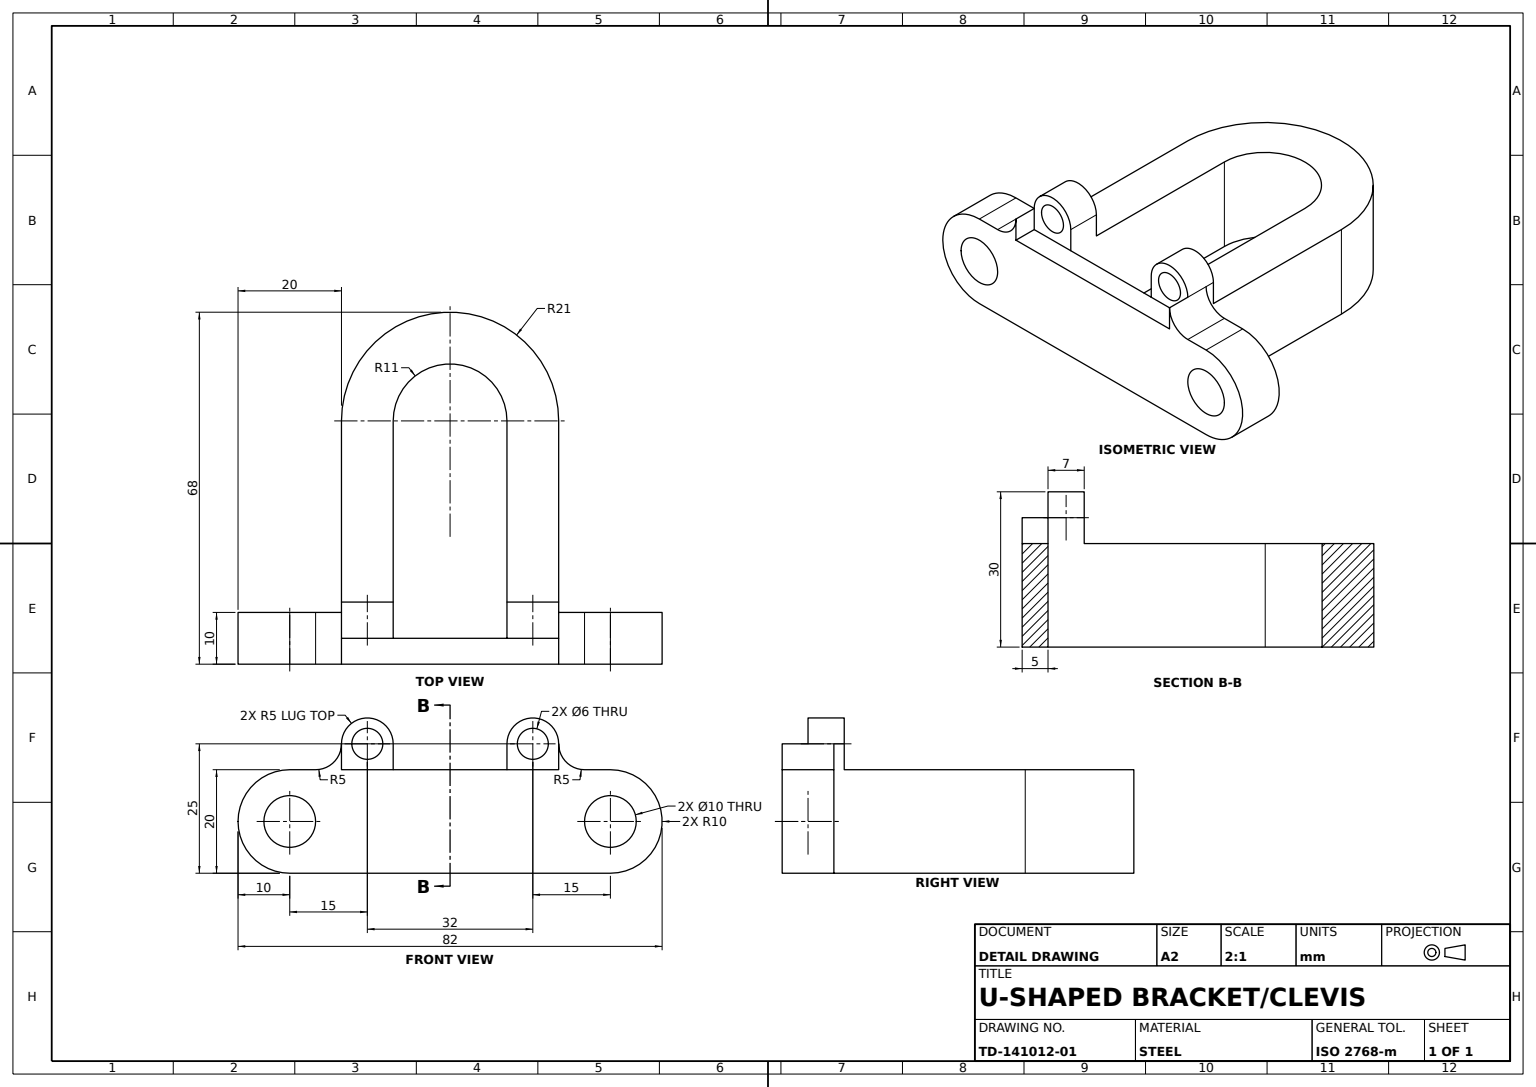
from build123d import *

# Parameters (mm, degrees)
BASE_PLATE_SKETCH_W    = 42
BASE_PLATE_SKETCH_H    = 20
BASE_PLATE_DEPTH       = 5
CURVED_LOOP_BOSS_DEPTH = 20
LOOP_SLOT_CUT_DEPTH    = 79.31347266
LUG_SKETCH_R           = 3
LUG_BOSS_DEPTH         = 7
PIN_EYE_SKETCH_R       = 5
PIN_EYE_BOSS_DEPTH     = 5


with BuildPart() as part:
    # Base Plate Sketch → Base Plate (new body)
    with BuildSketch(Plane.XY):
        with Locations((21, 10)):
            Rectangle(BASE_PLATE_SKETCH_W, BASE_PLATE_SKETCH_H)
    extrude(amount=BASE_PLATE_DEPTH)

    # Curved Loop Sketch → Curved Loop Boss (add, through all)
    with BuildSketch(Plane(origin=(0, 20, 0), x_dir=(1, 0, 0), z_dir=(0, 1, 0))):
        with BuildLine():
            Line((0, 42), (0, 0))
            Line((0, 0), (42, 0))
            Line((42, 0), (42, 42))
            ThreePointArc((42, 42), (21, 63), (0, 42))
        make_face()
    extrude(amount=-CURVED_LOOP_BOSS_DEPTH)

    # Loop Slot Sketch → Loop Slot Cut (cut, through all)
    with BuildSketch(Plane(origin=(0, 20, 0), x_dir=(1, 0, 0), z_dir=(0, 1, 0))):
        with BuildLine():
            Line((10, 42), (10, 0))
            Line((10, 0), (32, 0))
            Line((32, 0), (32, 42))
            ThreePointArc((32, 42), (21, 53), (10, 42))
        make_face()
    extrude(amount=-LOOP_SLOT_CUT_DEPTH, mode=Mode.SUBTRACT)

    # Lug Sketch → Lug Boss (add)
    with BuildSketch(Plane.XY):
        with BuildLine():
            Line((0, 25), (0, 20))
            Line((0, 20), (10, 20))
            Line((10, 20), (10, 25))
            ThreePointArc((10, 25), (5, 30), (0, 25))
        make_face()
        with Locations((5, 25)):
            Circle(LUG_SKETCH_R, mode=Mode.SUBTRACT)
    lug_boss = extrude(amount=-LUG_BOSS_DEPTH)

    # Lug Mirror: Lug Boss across plane
    add(lug_boss.mirror(Plane(origin=(21, 0, 0), x_dir=(0, 0, 1), z_dir=(1, 0, 0))))

    # Pin Eye Sketch → Pin Eye Boss (add, symmetric)
    with BuildSketch(Plane.XY):
        with BuildLine():
            Line((-10, 20), (-5, 20))
            ThreePointArc((-5, 20), (-1.464466094, 21.464466094), (0, 25))
            Line((0, 25), (0, 20))
            Line((0, 20), (0, 0))
            Line((0, 0), (-10, 0))
            ThreePointArc((-10, 0), (-20, 10), (-10, 20))
        make_face()
        with Locations((-10, 10)):
            Circle(PIN_EYE_SKETCH_R, mode=Mode.SUBTRACT)
    pin_eye_boss = extrude(amount=PIN_EYE_BOSS_DEPTH, both=True)

    # Pin Eye Mirror: Pin Eye Boss across plane
    add(pin_eye_boss.mirror(Plane(origin=(21, 0, 0), x_dir=(0, 0, 1), z_dir=(1, 0, 0))))


solid = part.part
